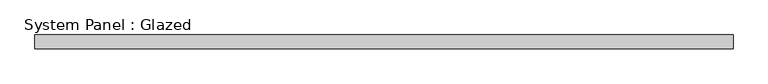
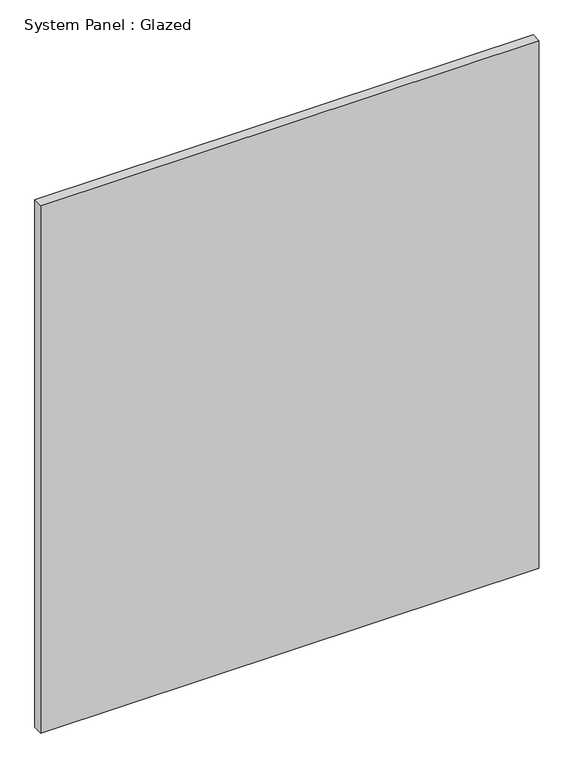
"""IFC4 building model written with IfcOpenShell, lengths in millimetres: plate geometry, System Panel : Glazed."""

from ifc_helpers import new_model, si_unit, origin, origin_with_axes, place, context, project, spatial, polyline, outline, extrude, source, transform, mapped, element, save


def system_panel_glazed_27c3d98e(model_context):
    return source(origin(), model_context, "Body", "SweptSolid", [
        extrude(outline(polyline([(638.175, 19.05), (-638.175, 19.05), (-638.175, 44.45), (638.175, 44.45), (638.175, 19.05)])), origin_with_axes(), (0.0, 0.0, 1.0), 1428.75),
    ])


if __name__ == "__main__":
    model = new_model("IFC4")
    model_context = context("Model", 3, world=origin())
    ifc_project = project(units=[si_unit("LENGTHUNIT", "METRE", prefix="MILLI")], contexts=[model_context])
    site = spatial("IfcSite", under=ifc_project)
    building = spatial("IfcBuilding", under=site)
    placement = place(None, origin())
    system_panel_glazed_shape = system_panel_glazed_27c3d98e(model_context)
    element("IfcPlate", 1, ObjectType="System Panel : Glazed", at=placement, inside=building, context=model_context, shape_type="MappedRepresentation", body=[
        mapped(system_panel_glazed_shape, transform((0.0, 0.0, 0.0), x_axis=(1.0, 0.0, 0.0), y_axis=(0.0, 1.0, 0.0), z_axis=(0.0, 0.0, 1.0))),
    ])
    save(model, "model.ifc")

# Revit data of these elements
# Type "System Panel : Glazed"
#   Construction Type Id = "GSP4R"
#   Analytic Construction = "1/8 in Pilkington single glazing"
#   Visual Light Transmittance = 0.9
#   Solar Heat Gain Coefficient = 0.86
#   Heat Transfer Coefficient (U) = 1.18115 BTU/(h·ft²·°F)
#   Define Thermal Properties by = 1
# Element 1 (IfcPlate, "System Panel : Glazed")
#   Materials on its faces: "Glass"
# Materials
#   "Glass": class "Glass", colour RGB 0 128 192, transparency 0.75, Description = "Soda Lime Glass", Cost = 0
